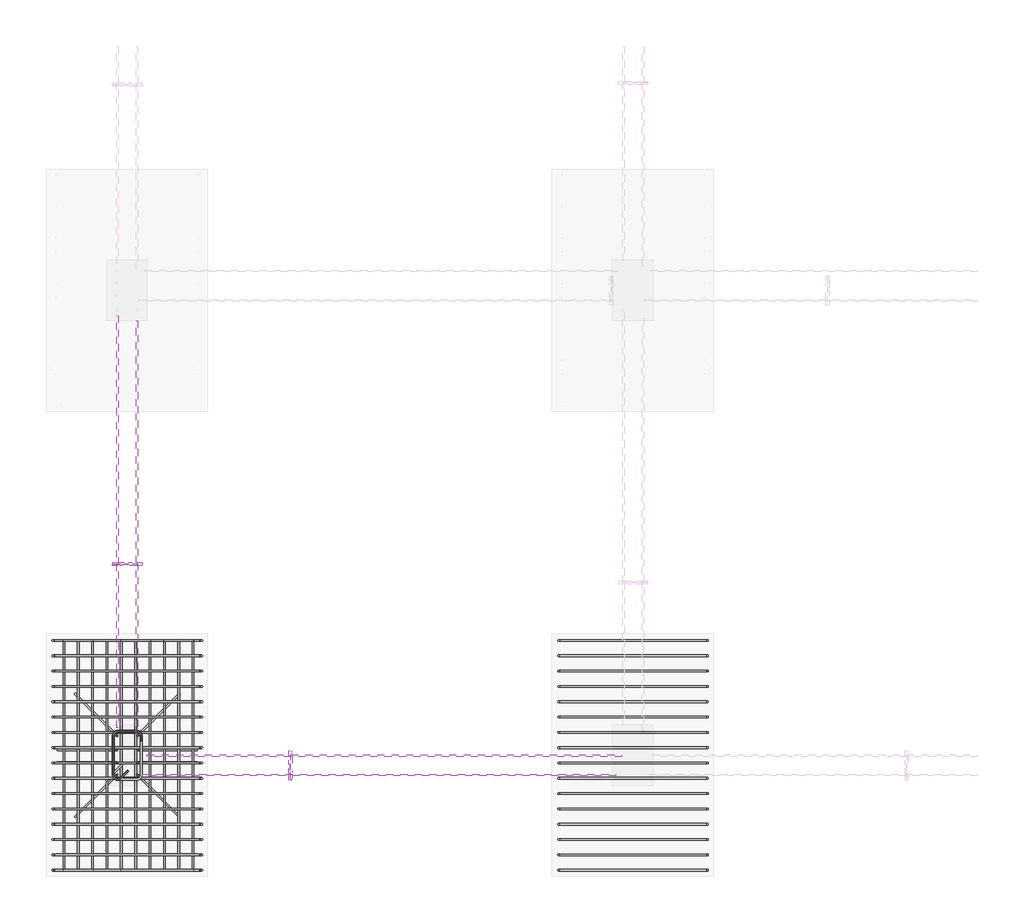
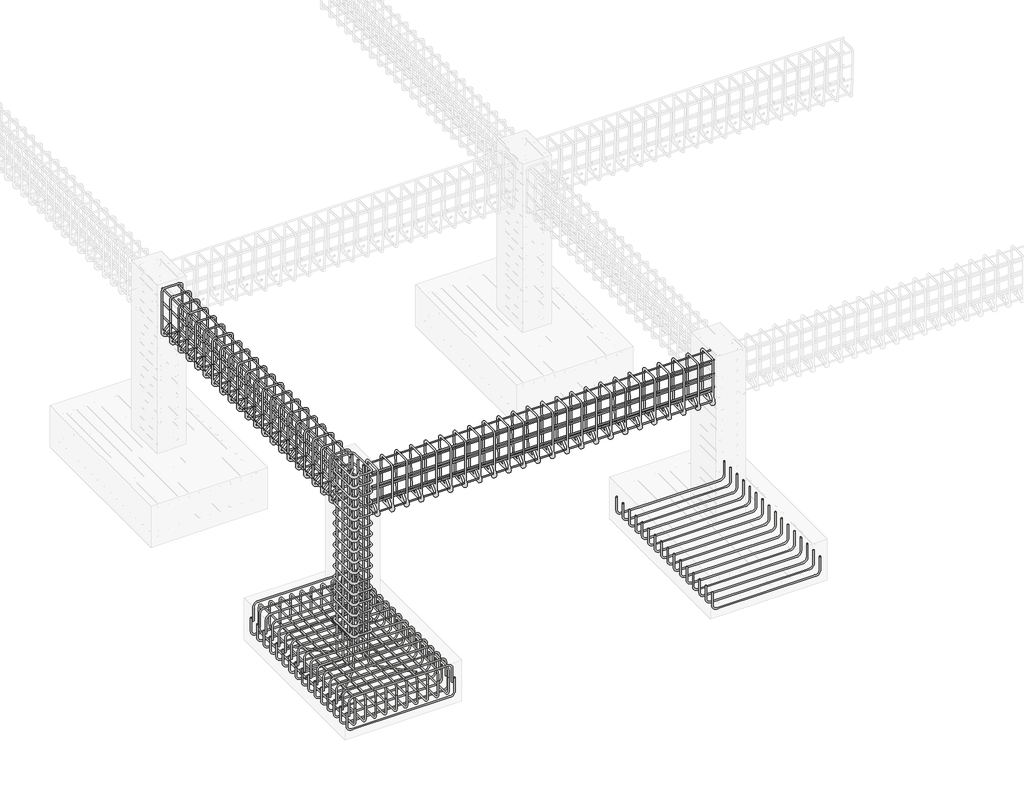
# One storey, part 2 of 20: 18 reinforcing bars.
"""IFC4 building model written with IfcOpenShell, lengths in millimetres."""

from ifc_helpers import new_model, si_unit, point, frame, origin, place, context, project, spatial, polyline, circle_curve, trimmed, segment, composite_curve, source, transform, mapped, element, save
from ifc_brep_helpers import swept_disk

model = new_model("IFC4")

# Units and contexts
model_context = context("Model", 3, world=origin())
ifc_project = project(units=[si_unit("LENGTHUNIT", "METRE", prefix="MILLI")], contexts=[model_context])

# Site, building, storey
site = spatial("IfcSite", under=ifc_project)
building = spatial("IfcBuilding", under=site)
storey = spatial("IfcBuildingStorey", under=building, Elevation=-1828.8)

# Reinforcing bars
placement = place(None, origin())
reinforcing_bar_shape = source(origin(), model_context, "Body", "SolidModel", [
    swept_disk(composite_curve([segment(polyline([(-6417.5912236, -7032.7168637, -2028.4704493), (-6417.5912236, -7032.7168637, -2175.7704493)]), True, "CONTINUOUS"), segment(trimmed(circle_curve(frame((-6371.2412236, -7032.7168637, -2175.7704493), z_axis=(0.0, -1.0, 0.0), x_axis=(-46.350000000000364, 0.0, 0.0)), 46.35), [point((-6417.5912236, -7032.7168637, -2175.7704493))], [point((-6371.2412236, -7032.7168637, -2222.1204493))], True, "CARTESIAN"), True, "CONTINUOUS"), segment(polyline([(-6371.2412236, -7032.7168637, -2222.1204493), (-5356.6412236, -7032.7168637, -2222.1204493)]), True, "CONTINUOUS"), segment(trimmed(circle_curve(frame((-5356.6412236, -7032.7168637, -2175.7704493), z_axis=(0.0, -1.0, 0.0), x_axis=(0.0, 0.0, -46.34999999999991)), 46.35), [point((-5356.6412236, -7032.7168637, -2222.1204493))], [point((-5310.2912236, -7032.7168637, -2175.7704493))], True, "CARTESIAN"), True, "CONTINUOUS"), segment(polyline([(-5310.2912236, -7032.7168637, -2175.7704493), (-5310.2912236, -7032.7168637, -2028.4704493)]), True, "CONTINUOUS")], self_intersect=False), 6.35),
])
element("IfcReinforcingBar", 1, at=placement, inside=storey, context=model_context, shape_type="MappedRepresentation", body=[
    mapped(reinforcing_bar_shape, transform((0.0, 0.0, 0.0), x_axis=(1.0, 0.0, 0.0), y_axis=(0.0, 1.0, 0.0), z_axis=(0.0, 0.0, 1.0))),
    mapped(reinforcing_bar_shape, transform((0.0, 113.82, 0.0), x_axis=(1.0, 0.0, 0.0), y_axis=(0.0, 1.0, 0.0), z_axis=(0.0, 0.0, 1.0))),
    mapped(reinforcing_bar_shape, transform((0.0, 227.64, 0.0), x_axis=(1.0, 0.0, 0.0), y_axis=(0.0, 1.0, 0.0), z_axis=(0.0, 0.0, 1.0))),
    mapped(reinforcing_bar_shape, transform((0.0, 341.46, 0.0), x_axis=(1.0, 0.0, 0.0), y_axis=(0.0, 1.0, 0.0), z_axis=(0.0, 0.0, 1.0))),
    mapped(reinforcing_bar_shape, transform((0.0, 455.28, 0.0), x_axis=(1.0, 0.0, 0.0), y_axis=(0.0, 1.0, 0.0), z_axis=(0.0, 0.0, 1.0))),
    mapped(reinforcing_bar_shape, transform((0.0, 569.1, 0.0), x_axis=(1.0, 0.0, 0.0), y_axis=(0.0, 1.0, 0.0), z_axis=(0.0, 0.0, 1.0))),
    mapped(reinforcing_bar_shape, transform((0.0, 682.92, 0.0), x_axis=(1.0, 0.0, 0.0), y_axis=(0.0, 1.0, 0.0), z_axis=(0.0, 0.0, 1.0))),
    mapped(reinforcing_bar_shape, transform((0.0, 796.74, 0.0), x_axis=(1.0, 0.0, 0.0), y_axis=(0.0, 1.0, 0.0), z_axis=(0.0, 0.0, 1.0))),
    mapped(reinforcing_bar_shape, transform((0.0, 910.56, 0.0), x_axis=(1.0, 0.0, 0.0), y_axis=(0.0, 1.0, 0.0), z_axis=(0.0, 0.0, 1.0))),
    mapped(reinforcing_bar_shape, transform((0.0, 1024.38, 0.0), x_axis=(1.0, 0.0, 0.0), y_axis=(0.0, 1.0, 0.0), z_axis=(0.0, 0.0, 1.0))),
    mapped(reinforcing_bar_shape, transform((0.0, 1138.2, 0.0), x_axis=(1.0, 0.0, 0.0), y_axis=(0.0, 1.0, 0.0), z_axis=(0.0, 0.0, 1.0))),
    mapped(reinforcing_bar_shape, transform((0.0, 1252.02, 0.0), x_axis=(1.0, 0.0, 0.0), y_axis=(0.0, 1.0, 0.0), z_axis=(0.0, 0.0, 1.0))),
    mapped(reinforcing_bar_shape, transform((0.0, 1365.84, 0.0), x_axis=(1.0, 0.0, 0.0), y_axis=(0.0, 1.0, 0.0), z_axis=(0.0, 0.0, 1.0))),
    mapped(reinforcing_bar_shape, transform((0.0, 1479.66, 0.0), x_axis=(1.0, 0.0, 0.0), y_axis=(0.0, 1.0, 0.0), z_axis=(0.0, 0.0, 1.0))),
    mapped(reinforcing_bar_shape, transform((0.0, 1593.48, 0.0), x_axis=(1.0, 0.0, 0.0), y_axis=(0.0, 1.0, 0.0), z_axis=(0.0, 0.0, 1.0))),
    mapped(reinforcing_bar_shape, transform((0.0, 1707.3, 0.0), x_axis=(1.0, 0.0, 0.0), y_axis=(0.0, 1.0, 0.0), z_axis=(0.0, 0.0, 1.0))),
])
reinforcing_bar_2_shape = source(origin(), model_context, "Body", "SolidModel", [
    swept_disk(composite_curve([segment(polyline([(-5334.4655685, -7032.7168637, -2068.8), (-5334.4655685, -7032.7168637, -1921.5)]), True, "CONTINUOUS"), segment(trimmed(circle_curve(frame((-5380.8155685, -7032.7168637, -1921.5), z_axis=(0.0, -1.0, 0.0), x_axis=(46.350000000000364, 0.0, 0.0)), 46.35), [point((-5334.4655685, -7032.7168637, -1921.5))], [point((-5380.8155685, -7032.7168637, -1875.15))], True, "CARTESIAN"), True, "CONTINUOUS"), segment(polyline([(-5380.8155685, -7032.7168637, -1875.15), (-6348.5369603, -7032.7168637, -1875.15)]), True, "CONTINUOUS"), segment(trimmed(circle_curve(frame((-6348.5369603, -7032.7168637, -1921.5), z_axis=(0.0, -1.0, 0.0), x_axis=(0.0, 0.0, 46.34999999999991)), 46.35), [point((-6348.5369603, -7032.7168637, -1875.15))], [point((-6394.8869603, -7032.7168637, -1921.5))], True, "CARTESIAN"), True, "CONTINUOUS"), segment(polyline([(-6394.8869603, -7032.7168637, -1921.5), (-6394.8869603, -7032.7168637, -2068.8)]), True, "CONTINUOUS")], self_intersect=False), 6.35),
])
element("IfcReinforcingBar", 2, at=placement, inside=storey, context=model_context, shape_type="MappedRepresentation", body=[
    mapped(reinforcing_bar_2_shape, transform((0.0, 0.0, 0.0), x_axis=(1.0, 0.0, 0.0), y_axis=(0.0, 1.0, 0.0), z_axis=(0.0, 0.0, 1.0))),
    mapped(reinforcing_bar_2_shape, transform((0.0, 113.82, 0.0), x_axis=(1.0, 0.0, 0.0), y_axis=(0.0, 1.0, 0.0), z_axis=(0.0, 0.0, 1.0))),
    mapped(reinforcing_bar_2_shape, transform((0.0, 227.64, 0.0), x_axis=(1.0, 0.0, 0.0), y_axis=(0.0, 1.0, 0.0), z_axis=(0.0, 0.0, 1.0))),
    mapped(reinforcing_bar_2_shape, transform((0.0, 341.46, 0.0), x_axis=(1.0, 0.0, 0.0), y_axis=(0.0, 1.0, 0.0), z_axis=(0.0, 0.0, 1.0))),
    mapped(reinforcing_bar_2_shape, transform((0.0, 455.28, 0.0), x_axis=(1.0, 0.0, 0.0), y_axis=(0.0, 1.0, 0.0), z_axis=(0.0, 0.0, 1.0))),
    mapped(reinforcing_bar_2_shape, transform((0.0, 569.1, 0.0), x_axis=(1.0, 0.0, 0.0), y_axis=(0.0, 1.0, 0.0), z_axis=(0.0, 0.0, 1.0))),
    mapped(reinforcing_bar_2_shape, transform((0.0, 682.92, 0.0), x_axis=(1.0, 0.0, 0.0), y_axis=(0.0, 1.0, 0.0), z_axis=(0.0, 0.0, 1.0))),
    mapped(reinforcing_bar_2_shape, transform((0.0, 796.74, 0.0), x_axis=(1.0, 0.0, 0.0), y_axis=(0.0, 1.0, 0.0), z_axis=(0.0, 0.0, 1.0))),
    mapped(reinforcing_bar_2_shape, transform((0.0, 910.56, 0.0), x_axis=(1.0, 0.0, 0.0), y_axis=(0.0, 1.0, 0.0), z_axis=(0.0, 0.0, 1.0))),
    mapped(reinforcing_bar_2_shape, transform((0.0, 1024.38, 0.0), x_axis=(1.0, 0.0, 0.0), y_axis=(0.0, 1.0, 0.0), z_axis=(0.0, 0.0, 1.0))),
    mapped(reinforcing_bar_2_shape, transform((0.0, 1138.2, 0.0), x_axis=(1.0, 0.0, 0.0), y_axis=(0.0, 1.0, 0.0), z_axis=(0.0, 0.0, 1.0))),
    mapped(reinforcing_bar_2_shape, transform((0.0, 1252.02, 0.0), x_axis=(1.0, 0.0, 0.0), y_axis=(0.0, 1.0, 0.0), z_axis=(0.0, 0.0, 1.0))),
    mapped(reinforcing_bar_2_shape, transform((0.0, 1365.84, 0.0), x_axis=(1.0, 0.0, 0.0), y_axis=(0.0, 1.0, 0.0), z_axis=(0.0, 0.0, 1.0))),
    mapped(reinforcing_bar_2_shape, transform((0.0, 1479.66, 0.0), x_axis=(1.0, 0.0, 0.0), y_axis=(0.0, 1.0, 0.0), z_axis=(0.0, 0.0, 1.0))),
    mapped(reinforcing_bar_2_shape, transform((0.0, 1593.48, 0.0), x_axis=(1.0, 0.0, 0.0), y_axis=(0.0, 1.0, 0.0), z_axis=(0.0, 0.0, 1.0))),
    mapped(reinforcing_bar_2_shape, transform((0.0, 1707.3, 0.0), x_axis=(1.0, 0.0, 0.0), y_axis=(0.0, 1.0, 0.0), z_axis=(0.0, 0.0, 1.0))),
])
reinforcing_bar_3_shape = source(origin(), model_context, "Body", "SolidModel", [
    swept_disk(composite_curve([segment(polyline([(-5374.0329187, -7032.7168637, -2008.6504502), (-5374.0329187, -7032.7168637, -2155.9504502)]), True, "CONTINUOUS"), segment(trimmed(circle_curve(frame((-5374.0329187, -6986.3668637, -2155.9504502), z_axis=(1.0, 0.0, 0.0), x_axis=(0.0, -46.350000000000364, 0.0)), 46.35), [point((-5374.0329187, -7032.7168637, -2155.9504502))], [point((-5374.0329187, -6986.3668637, -2202.3004502))], True, "CARTESIAN"), True, "CONTINUOUS"), segment(polyline([(-5374.0329187, -6986.3668637, -2202.3004502), (-5374.0329187, -5371.7668637, -2202.3004502)]), True, "CONTINUOUS"), segment(trimmed(circle_curve(frame((-5374.0329187, -5371.7668637, -2155.9504502), z_axis=(1.0, 0.0, 0.0), x_axis=(0.0, 0.0, -46.34999999999991)), 46.35), [point((-5374.0329187, -5371.7668637, -2202.3004502))], [point((-5374.0329187, -5325.4168637, -2155.9504502))], True, "CARTESIAN"), True, "CONTINUOUS"), segment(polyline([(-5374.0329187, -5325.4168637, -2155.9504502), (-5374.0329187, -5325.4168637, -2008.6504502)]), True, "CONTINUOUS")], self_intersect=False), 6.35),
])
element("IfcReinforcingBar", 3, at=placement, inside=storey, context=model_context, shape_type="MappedRepresentation", body=[
    mapped(reinforcing_bar_3_shape, transform((0.0, 0.0, 0.0), x_axis=(1.0, 0.0, 0.0), y_axis=(0.0, 1.0, 0.0), z_axis=(0.0, 0.0, 1.0))),
    mapped(reinforcing_bar_3_shape, transform((-106.7711398, 0.0, 0.0), x_axis=(1.0, 0.0, 0.0), y_axis=(0.0, 1.0, 0.0), z_axis=(0.0, 0.0, 1.0))),
    mapped(reinforcing_bar_3_shape, transform((-213.5422797, 0.0, 0.0), x_axis=(1.0, 0.0, 0.0), y_axis=(0.0, 1.0, 0.0), z_axis=(0.0, 0.0, 1.0))),
    mapped(reinforcing_bar_3_shape, transform((-320.3134195, 0.0, 0.0), x_axis=(1.0, 0.0, 0.0), y_axis=(0.0, 1.0, 0.0), z_axis=(0.0, 0.0, 1.0))),
    mapped(reinforcing_bar_3_shape, transform((-427.0845593, 0.0, 0.0), x_axis=(1.0, 0.0, 0.0), y_axis=(0.0, 1.0, 0.0), z_axis=(0.0, 0.0, 1.0))),
    mapped(reinforcing_bar_3_shape, transform((-533.8556992, 0.0, 0.0), x_axis=(1.0, 0.0, 0.0), y_axis=(0.0, 1.0, 0.0), z_axis=(0.0, 0.0, 1.0))),
    mapped(reinforcing_bar_3_shape, transform((-640.626839, 0.0, 0.0), x_axis=(1.0, 0.0, 0.0), y_axis=(0.0, 1.0, 0.0), z_axis=(0.0, 0.0, 1.0))),
    mapped(reinforcing_bar_3_shape, transform((-747.3979788, 0.0, 0.0), x_axis=(1.0, 0.0, 0.0), y_axis=(0.0, 1.0, 0.0), z_axis=(0.0, 0.0, 1.0))),
    mapped(reinforcing_bar_3_shape, transform((-854.1691187, 0.0, 0.0), x_axis=(1.0, 0.0, 0.0), y_axis=(0.0, 1.0, 0.0), z_axis=(0.0, 0.0, 1.0))),
    mapped(reinforcing_bar_3_shape, transform((-960.9402585, 0.0, 0.0), x_axis=(1.0, 0.0, 0.0), y_axis=(0.0, 1.0, 0.0), z_axis=(0.0, 0.0, 1.0))),
])
reinforcing_bar_4_shape = source(origin(), model_context, "Body", "SolidModel", [
    swept_disk(composite_curve([segment(polyline([(-6334.9731772, -7032.7168637, -2088.5147466), (-6334.9731772, -7032.7168637, -1941.2147466)]), True, "CONTINUOUS"), segment(trimmed(circle_curve(frame((-6334.9731772, -6986.3668637, -1941.2147466), z_axis=(-1.0, 0.0, 0.0), x_axis=(0.0, -46.350000000000364, 0.0)), 46.35), [point((-6334.9731772, -7032.7168637, -1941.2147466))], [point((-6334.9731772, -6986.3668637, -1894.8647466))], True, "CARTESIAN"), True, "CONTINUOUS"), segment(polyline([(-6334.9731772, -6986.3668637, -1894.8647466), (-6334.9731772, -5371.7668637, -1894.8647466)]), True, "CONTINUOUS"), segment(trimmed(circle_curve(frame((-6334.9731772, -5371.7668637, -1941.2147466), z_axis=(-1.0, 0.0, 0.0), x_axis=(0.0, 0.0, 46.34999999999991)), 46.35), [point((-6334.9731772, -5371.7668637, -1894.8647466))], [point((-6334.9731772, -5325.4168637, -1941.2147466))], True, "CARTESIAN"), True, "CONTINUOUS"), segment(polyline([(-6334.9731772, -5325.4168637, -1941.2147466), (-6334.9731772, -5325.4168637, -2088.5147466)]), True, "CONTINUOUS")], self_intersect=False), 6.35),
])
element("IfcReinforcingBar", 4, at=placement, inside=storey, context=model_context, shape_type="MappedRepresentation", body=[
    mapped(reinforcing_bar_4_shape, transform((0.0, 0.0, 0.0), x_axis=(1.0, 0.0, 0.0), y_axis=(0.0, 1.0, 0.0), z_axis=(0.0, 0.0, 1.0))),
    mapped(reinforcing_bar_4_shape, transform((106.7711398, 0.0, 0.0), x_axis=(1.0, 0.0, 0.0), y_axis=(0.0, 1.0, 0.0), z_axis=(0.0, 0.0, 1.0))),
    mapped(reinforcing_bar_4_shape, transform((213.5422797, 0.0, 0.0), x_axis=(1.0, 0.0, 0.0), y_axis=(0.0, 1.0, 0.0), z_axis=(0.0, 0.0, 1.0))),
    mapped(reinforcing_bar_4_shape, transform((320.3134195, 0.0, 0.0), x_axis=(1.0, 0.0, 0.0), y_axis=(0.0, 1.0, 0.0), z_axis=(0.0, 0.0, 1.0))),
    mapped(reinforcing_bar_4_shape, transform((427.0845593, 0.0, 0.0), x_axis=(1.0, 0.0, 0.0), y_axis=(0.0, 1.0, 0.0), z_axis=(0.0, 0.0, 1.0))),
    mapped(reinforcing_bar_4_shape, transform((533.8556992, 0.0, 0.0), x_axis=(1.0, 0.0, 0.0), y_axis=(0.0, 1.0, 0.0), z_axis=(0.0, 0.0, 1.0))),
    mapped(reinforcing_bar_4_shape, transform((640.626839, 0.0, 0.0), x_axis=(1.0, 0.0, 0.0), y_axis=(0.0, 1.0, 0.0), z_axis=(0.0, 0.0, 1.0))),
    mapped(reinforcing_bar_4_shape, transform((747.3979788, 0.0, 0.0), x_axis=(1.0, 0.0, 0.0), y_axis=(0.0, 1.0, 0.0), z_axis=(0.0, 0.0, 1.0))),
    mapped(reinforcing_bar_4_shape, transform((854.1691187, 0.0, 0.0), x_axis=(1.0, 0.0, 0.0), y_axis=(0.0, 1.0, 0.0), z_axis=(0.0, 0.0, 1.0))),
    mapped(reinforcing_bar_4_shape, transform((960.9402585, 0.0, 0.0), x_axis=(1.0, 0.0, 0.0), y_axis=(0.0, 1.0, 0.0), z_axis=(0.0, 0.0, 1.0))),
])
reinforcing_bar_5_shape = source(origin(), model_context, "Body", "SolidModel", [
    swept_disk(composite_curve([segment(polyline([(-2656.4360107, -7032.7168637, -2028.4704493), (-2656.4360107, -7032.7168637, -2175.7704493)]), True, "CONTINUOUS"), segment(trimmed(circle_curve(frame((-2610.0860107, -7032.7168637, -2175.7704493), z_axis=(0.0, -1.0, 0.0), x_axis=(-46.350000000000364, 0.0, 0.0)), 46.35), [point((-2656.4360107, -7032.7168637, -2175.7704493))], [point((-2610.0860107, -7032.7168637, -2222.1204493))], True, "CARTESIAN"), True, "CONTINUOUS"), segment(polyline([(-2610.0860107, -7032.7168637, -2222.1204493), (-1595.4860107, -7032.7168637, -2222.1204493)]), True, "CONTINUOUS"), segment(trimmed(circle_curve(frame((-1595.4860107, -7032.7168637, -2175.7704493), z_axis=(0.0, -1.0, 0.0), x_axis=(0.0, 0.0, -46.34999999999991)), 46.35), [point((-1595.4860107, -7032.7168637, -2222.1204493))], [point((-1549.1360107, -7032.7168637, -2175.7704493))], True, "CARTESIAN"), True, "CONTINUOUS"), segment(polyline([(-1549.1360107, -7032.7168637, -2175.7704493), (-1549.1360107, -7032.7168637, -2028.4704493)]), True, "CONTINUOUS")], self_intersect=False), 6.35),
])
element("IfcReinforcingBar", 5, at=placement, inside=storey, context=model_context, shape_type="MappedRepresentation", body=[
    mapped(reinforcing_bar_5_shape, transform((0.0, 0.0, 0.0), x_axis=(1.0, 0.0, 0.0), y_axis=(0.0, 1.0, 0.0), z_axis=(0.0, 0.0, 1.0))),
    mapped(reinforcing_bar_5_shape, transform((0.0, 113.82, 0.0), x_axis=(1.0, 0.0, 0.0), y_axis=(0.0, 1.0, 0.0), z_axis=(0.0, 0.0, 1.0))),
    mapped(reinforcing_bar_5_shape, transform((0.0, 227.64, 0.0), x_axis=(1.0, 0.0, 0.0), y_axis=(0.0, 1.0, 0.0), z_axis=(0.0, 0.0, 1.0))),
    mapped(reinforcing_bar_5_shape, transform((0.0, 341.46, 0.0), x_axis=(1.0, 0.0, 0.0), y_axis=(0.0, 1.0, 0.0), z_axis=(0.0, 0.0, 1.0))),
    mapped(reinforcing_bar_5_shape, transform((0.0, 455.28, 0.0), x_axis=(1.0, 0.0, 0.0), y_axis=(0.0, 1.0, 0.0), z_axis=(0.0, 0.0, 1.0))),
    mapped(reinforcing_bar_5_shape, transform((0.0, 569.1, 0.0), x_axis=(1.0, 0.0, 0.0), y_axis=(0.0, 1.0, 0.0), z_axis=(0.0, 0.0, 1.0))),
    mapped(reinforcing_bar_5_shape, transform((0.0, 682.92, 0.0), x_axis=(1.0, 0.0, 0.0), y_axis=(0.0, 1.0, 0.0), z_axis=(0.0, 0.0, 1.0))),
    mapped(reinforcing_bar_5_shape, transform((0.0, 796.74, 0.0), x_axis=(1.0, 0.0, 0.0), y_axis=(0.0, 1.0, 0.0), z_axis=(0.0, 0.0, 1.0))),
    mapped(reinforcing_bar_5_shape, transform((0.0, 910.56, 0.0), x_axis=(1.0, 0.0, 0.0), y_axis=(0.0, 1.0, 0.0), z_axis=(0.0, 0.0, 1.0))),
    mapped(reinforcing_bar_5_shape, transform((0.0, 1024.38, 0.0), x_axis=(1.0, 0.0, 0.0), y_axis=(0.0, 1.0, 0.0), z_axis=(0.0, 0.0, 1.0))),
    mapped(reinforcing_bar_5_shape, transform((0.0, 1138.2, 0.0), x_axis=(1.0, 0.0, 0.0), y_axis=(0.0, 1.0, 0.0), z_axis=(0.0, 0.0, 1.0))),
    mapped(reinforcing_bar_5_shape, transform((0.0, 1252.02, 0.0), x_axis=(1.0, 0.0, 0.0), y_axis=(0.0, 1.0, 0.0), z_axis=(0.0, 0.0, 1.0))),
    mapped(reinforcing_bar_5_shape, transform((0.0, 1365.84, 0.0), x_axis=(1.0, 0.0, 0.0), y_axis=(0.0, 1.0, 0.0), z_axis=(0.0, 0.0, 1.0))),
    mapped(reinforcing_bar_5_shape, transform((0.0, 1479.66, 0.0), x_axis=(1.0, 0.0, 0.0), y_axis=(0.0, 1.0, 0.0), z_axis=(0.0, 0.0, 1.0))),
    mapped(reinforcing_bar_5_shape, transform((0.0, 1593.48, 0.0), x_axis=(1.0, 0.0, 0.0), y_axis=(0.0, 1.0, 0.0), z_axis=(0.0, 0.0, 1.0))),
    mapped(reinforcing_bar_5_shape, transform((0.0, 1707.3, 0.0), x_axis=(1.0, 0.0, 0.0), y_axis=(0.0, 1.0, 0.0), z_axis=(0.0, 0.0, 1.0))),
])
reinforcing_bar_6_shape = source(origin(), model_context, "Body", "SolidModel", [
    swept_disk(composite_curve([segment(polyline([(-5858.3298631, -6292.7910983, -46.35), (-5914.073426, -6348.5346613, -46.35)]), True, "CONTINUOUS"), segment(trimmed(circle_curve(frame((-5936.2412236, -6326.3668637, -46.35), z_axis=(0.0, 0.0, -1.0), x_axis=(22.167797600000085, -22.167797600000085, 0.0)), 31.35), [point((-5914.073426, -6348.5346613, -46.35))], [point((-5967.5912236, -6326.3668637, -46.35))], True, "CARTESIAN"), True, "CONTINUOUS"), segment(polyline([(-5967.5912236, -6326.3668637, -46.35), (-5967.5912236, -6031.7668637, -46.35)]), True, "CONTINUOUS"), segment(trimmed(circle_curve(frame((-5936.2412236, -6031.7668637, -46.35), z_axis=(0.0, 0.0, -1.0), x_axis=(-31.350000000000364, 0.0, 0.0)), 31.35), [point((-5967.5912236, -6031.7668637, -46.35))], [point((-5936.2412236, -6000.4168637, -46.35))], True, "CARTESIAN"), True, "CONTINUOUS"), segment(polyline([(-5936.2412236, -6000.4168637, -46.35), (-5791.6412236, -6000.4168637, -46.35)]), True, "CONTINUOUS"), segment(trimmed(circle_curve(frame((-5791.6412236, -6031.7470786, -45.2363875), z_axis=(0.0, -0.035521928334481916, -0.9993688971583016), x_axis=(0.0, 31.3302149000001, -1.1136125000000021)), 31.35), [point((-5791.6412236, -6000.4168637, -46.35))], [point((-5760.2912236, -6031.7470786, -45.2363875))], True, "CARTESIAN"), True, "CONTINUOUS"), segment(polyline([(-5760.2912236, -6031.7470786, -45.2363875), (-5760.2912236, -6326.3866488, -34.7636125)]), True, "CONTINUOUS"), segment(trimmed(circle_curve(frame((-5791.6412236, -6326.3866488, -34.7636125), z_axis=(0.0, -0.035521928334481916, -0.9993688971583016), x_axis=(31.349999999999454, 0.0, 0.0)), 31.35), [point((-5760.2912236, -6326.3866488, -34.7636125))], [point((-5791.6412236, -6357.7168637, -33.65))], True, "CARTESIAN"), True, "CONTINUOUS"), segment(polyline([(-5791.6412236, -6357.7168637, -33.65), (-5936.2412236, -6357.7168637, -33.65)]), True, "CONTINUOUS"), segment(trimmed(circle_curve(frame((-5936.2412236, -6326.3668637, -33.65), z_axis=(0.0, 0.0, -1.0), x_axis=(0.0, -31.350000000000364, 0.0)), 31.35), [point((-5936.2412236, -6357.7168637, -33.65))], [point((-5958.4090212, -6304.1990661, -33.65))], True, "CARTESIAN"), True, "CONTINUOUS"), segment(polyline([(-5958.4090212, -6304.1990661, -33.65), (-5902.6654583, -6248.4555031, -33.65)]), True, "CONTINUOUS")], self_intersect=False), 6.35),
])
element("IfcReinforcingBar", 6, at=placement, inside=storey, context=model_context, shape_type="MappedRepresentation", body=[
    mapped(reinforcing_bar_6_shape, transform((0.0, 0.0, 0.0), x_axis=(1.0, 0.0, 0.0), y_axis=(0.0, 1.0, 0.0), z_axis=(0.0, 0.0, 1.0))),
    mapped(reinforcing_bar_6_shape, transform((0.0, 0.0, -115.74), x_axis=(1.0, 0.0, 0.0), y_axis=(0.0, 1.0, 0.0), z_axis=(0.0, 0.0, 1.0))),
    mapped(reinforcing_bar_6_shape, transform((0.0, 0.0, -231.48), x_axis=(1.0, 0.0, 0.0), y_axis=(0.0, 1.0, 0.0), z_axis=(0.0, 0.0, 1.0))),
    mapped(reinforcing_bar_6_shape, transform((0.0, 0.0, -347.22), x_axis=(1.0, 0.0, 0.0), y_axis=(0.0, 1.0, 0.0), z_axis=(0.0, 0.0, 1.0))),
    mapped(reinforcing_bar_6_shape, transform((0.0, 0.0, -462.96), x_axis=(1.0, 0.0, 0.0), y_axis=(0.0, 1.0, 0.0), z_axis=(0.0, 0.0, 1.0))),
    mapped(reinforcing_bar_6_shape, transform((0.0, 0.0, -578.7), x_axis=(1.0, 0.0, 0.0), y_axis=(0.0, 1.0, 0.0), z_axis=(0.0, 0.0, 1.0))),
    mapped(reinforcing_bar_6_shape, transform((0.0, 0.0, -694.44), x_axis=(1.0, 0.0, 0.0), y_axis=(0.0, 1.0, 0.0), z_axis=(0.0, 0.0, 1.0))),
    mapped(reinforcing_bar_6_shape, transform((0.0, 0.0, -810.18), x_axis=(1.0, 0.0, 0.0), y_axis=(0.0, 1.0, 0.0), z_axis=(0.0, 0.0, 1.0))),
    mapped(reinforcing_bar_6_shape, transform((0.0, 0.0, -925.92), x_axis=(1.0, 0.0, 0.0), y_axis=(0.0, 1.0, 0.0), z_axis=(0.0, 0.0, 1.0))),
    mapped(reinforcing_bar_6_shape, transform((0.0, 0.0, -1041.66), x_axis=(1.0, 0.0, 0.0), y_axis=(0.0, 1.0, 0.0), z_axis=(0.0, 0.0, 1.0))),
    mapped(reinforcing_bar_6_shape, transform((0.0, 0.0, -1157.4), x_axis=(1.0, 0.0, 0.0), y_axis=(0.0, 1.0, 0.0), z_axis=(0.0, 0.0, 1.0))),
    mapped(reinforcing_bar_6_shape, transform((0.0, 0.0, -1273.14), x_axis=(1.0, 0.0, 0.0), y_axis=(0.0, 1.0, 0.0), z_axis=(0.0, 0.0, 1.0))),
    mapped(reinforcing_bar_6_shape, transform((0.0, 0.0, -1388.88), x_axis=(1.0, 0.0, 0.0), y_axis=(0.0, 1.0, 0.0), z_axis=(0.0, 0.0, 1.0))),
    mapped(reinforcing_bar_6_shape, transform((0.0, 0.0, -1504.62), x_axis=(1.0, 0.0, 0.0), y_axis=(0.0, 1.0, 0.0), z_axis=(0.0, 0.0, 1.0))),
    mapped(reinforcing_bar_6_shape, transform((0.0, 0.0, -1620.36), x_axis=(1.0, 0.0, 0.0), y_axis=(0.0, 1.0, 0.0), z_axis=(0.0, 0.0, 1.0))),
    mapped(reinforcing_bar_6_shape, transform((0.0, 0.0, -1736.1), x_axis=(1.0, 0.0, 0.0), y_axis=(0.0, 1.0, 0.0), z_axis=(0.0, 0.0, 1.0))),
])
reinforcing_bar_7_shape = source(origin(), model_context, "Body", "SolidModel", [
    swept_disk(composite_curve([segment(polyline([(-5343.4123372, -6232.7428863, -2151.8747939), (-5740.4296686, -6232.7428863, -2151.8747939)]), True, "CONTINUOUS"), segment(trimmed(circle_curve(frame((-5740.4296686, -6232.7428863, -2105.5247939), z_axis=(0.0, 1.0, 0.0), x_axis=(0.0, 0.0, -46.34999999999991)), 46.35), [point((-5740.4296686, -6232.7428863, -2151.8747939))], [point((-5786.7796686, -6232.7428863, -2105.5247939))], True, "CARTESIAN"), True, "CONTINUOUS"), segment(polyline([(-5786.7796686, -6232.7428863, -2105.5247939), (-5786.7796686, -6232.7428863, -40.0)]), True, "CONTINUOUS")], self_intersect=False), 6.35),
])
element("IfcReinforcingBar", 7, at=placement, inside=storey, context=model_context, shape_type="MappedRepresentation", body=[
    mapped(reinforcing_bar_7_shape, transform((0.0, 0.0, 0.0), x_axis=(1.0, 0.0, 0.0), y_axis=(0.0, 1.0, 0.0), z_axis=(0.0, 0.0, 1.0))),
    mapped(reinforcing_bar_7_shape, transform((0.0, 93.9182821, 0.0), x_axis=(1.0, 0.0, 0.0), y_axis=(0.0, 1.0, 0.0), z_axis=(0.0, 0.0, 1.0))),
])
element("IfcReinforcingBar", 8, at=placement, inside=storey, context=model_context, shape_type="SolidModel", body=[
    swept_disk(composite_curve([segment(polyline([(-5473.271622, -5719.5629186, -2151.8747939), (-5754.0052693, -6000.2965659, -2151.8747939)]), True, "CONTINUOUS"), segment(trimmed(circle_curve(frame((-5754.0052693, -6000.2965659, -2105.5247939), z_axis=(-0.7071067811865442, 0.7071067811865509, 0.0), x_axis=(0.0, 0.0, -46.34999999999991)), 46.35), [point((-5754.0052693, -6000.2965659, -2151.8747939))], [point((-5786.7796686, -6033.0709652, -2105.5247939))], True, "CARTESIAN"), True, "CONTINUOUS"), segment(polyline([(-5786.7796686, -6033.0709652, -2105.5247939), (-5786.7796686, -6033.0709652, -40.0)]), True, "CONTINUOUS")], self_intersect=False), 6.35),
])
element("IfcReinforcingBar", 9, at=placement, inside=storey, context=model_context, shape_type="SolidModel", body=[
    swept_disk(composite_curve([segment(polyline([(-6254.6108252, -5719.5629186, -2151.8747939), (-5973.877178, -6000.2965659, -2151.8747939)]), True, "CONTINUOUS"), segment(trimmed(circle_curve(frame((-5973.877178, -6000.2965659, -2105.5247939), z_axis=(-0.7071067811865442, -0.7071067811865509, 0.0), x_axis=(0.0, 0.0, -46.34999999999991)), 46.35), [point((-5973.877178, -6000.2965659, -2151.8747939))], [point((-5941.1027787, -6033.0709652, -2105.5247939))], True, "CARTESIAN"), True, "CONTINUOUS"), segment(polyline([(-5941.1027787, -6033.0709652, -2105.5247939), (-5941.1027787, -6033.0709652, -40.0)]), True, "CONTINUOUS")], self_intersect=False), 6.35),
])
element("IfcReinforcingBar", 10, at=placement, inside=storey, context=model_context, shape_type="SolidModel", body=[
    swept_disk(composite_curve([segment(polyline([(-5473.271622, -6638.5708088, -2151.8747939), (-5754.0052693, -6357.8371615, -2151.8747939)]), True, "CONTINUOUS"), segment(trimmed(circle_curve(frame((-5754.0052693, -6357.8371615, -2105.5247939), z_axis=(0.7071067811865442, 0.7071067811865509, 0.0), x_axis=(0.0, 0.0, -46.34999999999991)), 46.35), [point((-5754.0052693, -6357.8371615, -2151.8747939))], [point((-5786.7796686, -6325.0627622, -2105.5247939))], True, "CARTESIAN"), True, "CONTINUOUS"), segment(polyline([(-5786.7796686, -6325.0627622, -2105.5247939), (-5786.7796686, -6325.0627622, -40.0)]), True, "CONTINUOUS")], self_intersect=False), 6.35),
])
element("IfcReinforcingBar", 11, at=placement, inside=storey, context=model_context, shape_type="SolidModel", body=[
    swept_disk(composite_curve([segment(polyline([(-6254.6108252, -6638.5708088, -2151.8747939), (-5973.877178, -6357.8371615, -2151.8747939)]), True, "CONTINUOUS"), segment(trimmed(circle_curve(frame((-5973.877178, -6357.8371615, -2105.5247939), z_axis=(0.7071067811865442, -0.7071067811865509, 0.0), x_axis=(0.0, 0.0, -46.34999999999991)), 46.35), [point((-5973.877178, -6357.8371615, -2151.8747939))], [point((-5941.1027787, -6325.0627622, -2105.5247939))], True, "CARTESIAN"), True, "CONTINUOUS"), segment(polyline([(-5941.1027787, -6325.0627622, -2105.5247939), (-5941.1027787, -6325.0627622, -40.0)]), True, "CONTINUOUS")], self_intersect=False), 6.35),
])
reinforcing_bar_8_shape = source(origin(), model_context, "Body", "SolidModel", [
    swept_disk(composite_curve([segment(polyline([(-6384.4701101, -6232.7428863, -2151.8747939), (-5987.4527787, -6232.7428863, -2151.8747939)]), True, "CONTINUOUS"), segment(trimmed(circle_curve(frame((-5987.4527787, -6232.7428863, -2105.5247939), z_axis=(0.0, -1.0, 0.0), x_axis=(0.0, 0.0, -46.34999999999991)), 46.35), [point((-5987.4527787, -6232.7428863, -2151.8747939))], [point((-5941.1027787, -6232.7428863, -2105.5247939))], True, "CARTESIAN"), True, "CONTINUOUS"), segment(polyline([(-5941.1027787, -6232.7428863, -2105.5247939), (-5941.1027787, -6232.7428863, -40.0)]), True, "CONTINUOUS")], self_intersect=False), 6.35),
])
element("IfcReinforcingBar", 12, at=placement, inside=storey, context=model_context, shape_type="MappedRepresentation", body=[
    mapped(reinforcing_bar_8_shape, transform((0.0, 0.0, 0.0), x_axis=(1.0, 0.0, 0.0), y_axis=(0.0, 1.0, 0.0), z_axis=(0.0, 0.0, 1.0))),
    mapped(reinforcing_bar_8_shape, transform((0.0, 93.9182821, 0.0), x_axis=(1.0, 0.0, 0.0), y_axis=(0.0, 1.0, 0.0), z_axis=(0.0, 0.0, 1.0))),
])
reinforcing_bar_9_shape = source(origin(), model_context, "Body", "SolidModel", [
    swept_disk(composite_curve([segment(polyline([(-5858.3298631, -5947.7168643, -488.7242346), (-5914.073426, -5947.7168643, -544.4677976)]), True, "CONTINUOUS"), segment(trimmed(circle_curve(frame((-5936.2412236, -5947.7168643, -522.3), z_axis=(0.0, 1.0, 0.0), x_axis=(22.167797600000085, 0.0, -22.167797600000085)), 31.35), [point((-5914.073426, -5947.7168643, -544.4677976))], [point((-5967.5912236, -5947.7168643, -522.3))], True, "CARTESIAN"), True, "CONTINUOUS"), segment(polyline([(-5967.5912236, -5947.7168643, -522.3), (-5967.5912236, -5947.7168643, -77.7)]), True, "CONTINUOUS"), segment(trimmed(circle_curve(frame((-5936.2412236, -5947.7168643, -77.7), z_axis=(0.0, 1.0, 0.0), x_axis=(-31.350000000000364, 0.0, 0.0)), 31.35), [point((-5967.5912236, -5947.7168643, -77.7))], [point((-5936.2412236, -5947.7168643, -46.35))], True, "CARTESIAN"), True, "CONTINUOUS"), segment(polyline([(-5936.2412236, -5947.7168643, -46.35), (-5791.6412236, -5947.7168643, -46.35)]), True, "CONTINUOUS"), segment(trimmed(circle_curve(frame((-5791.6412236, -5948.5014499, -77.6901807), z_axis=(0.0, 0.9996867842138424, -0.025026655153786322), x_axis=(0.0, 0.7845855999994455, 31.340180699999998)), 31.35), [point((-5791.6412236, -5947.7168643, -46.35))], [point((-5760.2912236, -5948.5014499, -77.6901807))], True, "CARTESIAN"), True, "CONTINUOUS"), segment(polyline([(-5760.2912236, -5948.5014499, -77.6901807), (-5760.2912236, -5959.6322786, -522.3098193)]), True, "CONTINUOUS"), segment(trimmed(circle_curve(frame((-5791.6412236, -5959.6322786, -522.3098193), z_axis=(0.0, 0.9996867842138424, -0.025026655153786322), x_axis=(31.349999999999454, 0.0, 0.0)), 31.35), [point((-5760.2912236, -5959.6322786, -522.3098193))], [point((-5791.6412236, -5960.4168643, -553.65))], True, "CARTESIAN"), True, "CONTINUOUS"), segment(polyline([(-5791.6412236, -5960.4168643, -553.65), (-5936.2412236, -5960.4168643, -553.65)]), True, "CONTINUOUS"), segment(trimmed(circle_curve(frame((-5936.2412236, -5960.4168643, -522.3), z_axis=(0.0, 1.0, 0.0), x_axis=(0.0, 0.0, -31.350000000000023)), 31.35), [point((-5936.2412236, -5960.4168643, -553.65))], [point((-5958.4090212, -5960.4168643, -500.1322024))], True, "CARTESIAN"), True, "CONTINUOUS"), segment(polyline([(-5958.4090212, -5960.4168643, -500.1322024), (-5902.6654583, -5960.4168643, -444.3886395)]), True, "CONTINUOUS")], self_intersect=False), 6.35),
])
element("IfcReinforcingBar", 13, at=placement, inside=storey, context=model_context, shape_type="MappedRepresentation", body=[
    mapped(reinforcing_bar_9_shape, transform((0.0, 0.0, 0.0), x_axis=(1.0, 0.0, 0.0), y_axis=(0.0, 1.0, 0.0), z_axis=(0.0, 0.0, 1.0))),
    mapped(reinforcing_bar_9_shape, transform((0.0, 149.585, 0.0), x_axis=(1.0, 0.0, 0.0), y_axis=(0.0, 1.0, 0.0), z_axis=(0.0, 0.0, 1.0))),
    mapped(reinforcing_bar_9_shape, transform((0.0, 299.1700001, 0.0), x_axis=(1.0, 0.0, 0.0), y_axis=(0.0, 1.0, 0.0), z_axis=(0.0, 0.0, 1.0))),
    mapped(reinforcing_bar_9_shape, transform((0.0, 448.7550001, 0.0), x_axis=(1.0, 0.0, 0.0), y_axis=(0.0, 1.0, 0.0), z_axis=(0.0, 0.0, 1.0))),
    mapped(reinforcing_bar_9_shape, transform((0.0, 598.3400001, 0.0), x_axis=(1.0, 0.0, 0.0), y_axis=(0.0, 1.0, 0.0), z_axis=(0.0, 0.0, 1.0))),
    mapped(reinforcing_bar_9_shape, transform((0.0, 747.9250002, 0.0), x_axis=(1.0, 0.0, 0.0), y_axis=(0.0, 1.0, 0.0), z_axis=(0.0, 0.0, 1.0))),
    mapped(reinforcing_bar_9_shape, transform((0.0, 897.5100002, 0.0), x_axis=(1.0, 0.0, 0.0), y_axis=(0.0, 1.0, 0.0), z_axis=(0.0, 0.0, 1.0))),
    mapped(reinforcing_bar_9_shape, transform((0.0, 1047.0950002, 0.0), x_axis=(1.0, 0.0, 0.0), y_axis=(0.0, 1.0, 0.0), z_axis=(0.0, 0.0, 1.0))),
    mapped(reinforcing_bar_9_shape, transform((0.0, 1196.6800002, 0.0), x_axis=(1.0, 0.0, 0.0), y_axis=(0.0, 1.0, 0.0), z_axis=(0.0, 0.0, 1.0))),
    mapped(reinforcing_bar_9_shape, transform((0.0, 1346.2650003, 0.0), x_axis=(1.0, 0.0, 0.0), y_axis=(0.0, 1.0, 0.0), z_axis=(0.0, 0.0, 1.0))),
    mapped(reinforcing_bar_9_shape, transform((0.0, 1495.8500003, 0.0), x_axis=(1.0, 0.0, 0.0), y_axis=(0.0, 1.0, 0.0), z_axis=(0.0, 0.0, 1.0))),
    mapped(reinforcing_bar_9_shape, transform((0.0, 1645.4350003, 0.0), x_axis=(1.0, 0.0, 0.0), y_axis=(0.0, 1.0, 0.0), z_axis=(0.0, 0.0, 1.0))),
    mapped(reinforcing_bar_9_shape, transform((0.0, 1795.0200004, 0.0), x_axis=(1.0, 0.0, 0.0), y_axis=(0.0, 1.0, 0.0), z_axis=(0.0, 0.0, 1.0))),
    mapped(reinforcing_bar_9_shape, transform((0.0, 1944.6050004, 0.0), x_axis=(1.0, 0.0, 0.0), y_axis=(0.0, 1.0, 0.0), z_axis=(0.0, 0.0, 1.0))),
    mapped(reinforcing_bar_9_shape, transform((0.0, 2094.1900004, 0.0), x_axis=(1.0, 0.0, 0.0), y_axis=(0.0, 1.0, 0.0), z_axis=(0.0, 0.0, 1.0))),
    mapped(reinforcing_bar_9_shape, transform((0.0, 2243.7750005, 0.0), x_axis=(1.0, 0.0, 0.0), y_axis=(0.0, 1.0, 0.0), z_axis=(0.0, 0.0, 1.0))),
    mapped(reinforcing_bar_9_shape, transform((0.0, 2393.3600005, 0.0), x_axis=(1.0, 0.0, 0.0), y_axis=(0.0, 1.0, 0.0), z_axis=(0.0, 0.0, 1.0))),
    mapped(reinforcing_bar_9_shape, transform((0.0, 2542.9450005, 0.0), x_axis=(1.0, 0.0, 0.0), y_axis=(0.0, 1.0, 0.0), z_axis=(0.0, 0.0, 1.0))),
    mapped(reinforcing_bar_9_shape, transform((0.0, 2692.5300005, 0.0), x_axis=(1.0, 0.0, 0.0), y_axis=(0.0, 1.0, 0.0), z_axis=(0.0, 0.0, 1.0))),
    mapped(reinforcing_bar_9_shape, transform((0.0, 2842.1150006, 0.0), x_axis=(1.0, 0.0, 0.0), y_axis=(0.0, 1.0, 0.0), z_axis=(0.0, 0.0, 1.0))),
    mapped(reinforcing_bar_9_shape, transform((0.0, 2991.7000006, 0.0), x_axis=(1.0, 0.0, 0.0), y_axis=(0.0, 1.0, 0.0), z_axis=(0.0, 0.0, 1.0))),
])
reinforcing_bar_10_shape = source(origin(), model_context, "Body", "SolidModel", [
    swept_disk(composite_curve([segment(polyline([(-5936.2412236, -5975.1202711, -522.0844), (-5936.2412236, -2909.6668637, -522.0844)]), True, "CONTINUOUS")], self_intersect=False), 6.35),
])
element("IfcReinforcingBar", 14, at=placement, inside=storey, context=model_context, shape_type="MappedRepresentation", body=[
    mapped(reinforcing_bar_10_shape, transform((0.0, 0.0, 0.0), x_axis=(1.0, 0.0, 0.0), y_axis=(0.0, 1.0, 0.0), z_axis=(0.0, 0.0, 1.0))),
    mapped(reinforcing_bar_10_shape, transform((0.0, 0.0, 147.799393), x_axis=(1.0, 0.0, 0.0), y_axis=(0.0, 1.0, 0.0), z_axis=(0.0, 0.0, 1.0))),
    mapped(reinforcing_bar_10_shape, transform((0.0, 0.0, 295.598786), x_axis=(1.0, 0.0, 0.0), y_axis=(0.0, 1.0, 0.0), z_axis=(0.0, 0.0, 1.0))),
    mapped(reinforcing_bar_10_shape, transform((0.0, 0.0, 443.398179), x_axis=(1.0, 0.0, 0.0), y_axis=(0.0, 1.0, 0.0), z_axis=(0.0, 0.0, 1.0))),
])
reinforcing_bar_11_shape = source(origin(), model_context, "Body", "SolidModel", [
    swept_disk(composite_curve([segment(polyline([(-5791.6412236, -6019.1737816, -522.0844), (-5791.6412236, -2948.4810721, -522.0844)]), True, "CONTINUOUS")], self_intersect=False), 6.35),
])
element("IfcReinforcingBar", 15, at=placement, inside=storey, context=model_context, shape_type="MappedRepresentation", body=[
    mapped(reinforcing_bar_11_shape, transform((0.0, 0.0, 0.0), x_axis=(1.0, 0.0, 0.0), y_axis=(0.0, 1.0, 0.0), z_axis=(0.0, 0.0, 1.0))),
    mapped(reinforcing_bar_11_shape, transform((0.0, 0.0, 147.799393), x_axis=(1.0, 0.0, 0.0), y_axis=(0.0, 1.0, 0.0), z_axis=(0.0, 0.0, 1.0))),
    mapped(reinforcing_bar_11_shape, transform((0.0, 0.0, 295.598786), x_axis=(1.0, 0.0, 0.0), y_axis=(0.0, 1.0, 0.0), z_axis=(0.0, 0.0, 1.0))),
    mapped(reinforcing_bar_11_shape, transform((0.0, 0.0, 443.398179), x_axis=(1.0, 0.0, 0.0), y_axis=(0.0, 1.0, 0.0), z_axis=(0.0, 0.0, 1.0))),
])
reinforcing_bar_12_shape = source(origin(), model_context, "Body", "SolidModel", [
    swept_disk(composite_curve([segment(polyline([(-2259.1360107, -6248.4555031, -488.7242346), (-2259.1360107, -6304.1990661, -544.4677976)]), True, "CONTINUOUS"), segment(trimmed(circle_curve(frame((-2259.1360107, -6326.3668637, -522.3), z_axis=(-1.0, 0.0, 0.0), x_axis=(0.0, 22.167797600000085, -22.167797600000085)), 31.35), [point((-2259.1360107, -6304.1990661, -544.4677976))], [point((-2259.1360107, -6357.7168637, -522.3))], True, "CARTESIAN"), True, "CONTINUOUS"), segment(polyline([(-2259.1360107, -6357.7168637, -522.3), (-2259.1360107, -6357.7168637, -77.7)]), True, "CONTINUOUS"), segment(trimmed(circle_curve(frame((-2259.1360107, -6326.3668637, -77.7), z_axis=(-1.0, 0.0, 0.0), x_axis=(0.0, -31.350000000000364, 0.0)), 31.35), [point((-2259.1360107, -6357.7168637, -77.7))], [point((-2259.1360107, -6326.3668637, -46.35))], True, "CARTESIAN"), True, "CONTINUOUS"), segment(polyline([(-2259.1360107, -6326.3668637, -46.35), (-2259.1360107, -6181.7668637, -46.35)]), True, "CONTINUOUS"), segment(trimmed(circle_curve(frame((-2258.3514251, -6181.7668637, -77.6901807), z_axis=(-0.9996867842138424, 0.0, -0.025026655153786322), x_axis=(-0.7845855999999003, 0.0, 31.340180699999998)), 31.35), [point((-2259.1360107, -6181.7668637, -46.35))], [point((-2258.3514251, -6150.4168637, -77.6901807))], True, "CARTESIAN"), True, "CONTINUOUS"), segment(polyline([(-2258.3514251, -6150.4168637, -77.6901807), (-2247.2205963, -6150.4168637, -522.3098193)]), True, "CONTINUOUS"), segment(trimmed(circle_curve(frame((-2247.2205963, -6181.7668637, -522.3098193), z_axis=(-0.9996867842138424, 0.0, -0.025026655153786322), x_axis=(0.0, 31.349999999999454, 0.0)), 31.35), [point((-2247.2205963, -6150.4168637, -522.3098193))], [point((-2246.4360107, -6181.7668637, -553.65))], True, "CARTESIAN"), True, "CONTINUOUS"), segment(polyline([(-2246.4360107, -6181.7668637, -553.65), (-2246.4360107, -6326.3668637, -553.65)]), True, "CONTINUOUS"), segment(trimmed(circle_curve(frame((-2246.4360107, -6326.3668637, -522.3), z_axis=(-1.0, 0.0, 0.0), x_axis=(0.0, 0.0, -31.350000000000023)), 31.35), [point((-2246.4360107, -6326.3668637, -553.65))], [point((-2246.4360107, -6348.5346613, -500.1322024))], True, "CARTESIAN"), True, "CONTINUOUS"), segment(polyline([(-2246.4360107, -6348.5346613, -500.1322024), (-2246.4360107, -6292.7910983, -444.3886395)]), True, "CONTINUOUS")], self_intersect=False), 6.35),
])
element("IfcReinforcingBar", 16, at=placement, inside=storey, context=model_context, shape_type="MappedRepresentation", body=[
    mapped(reinforcing_bar_12_shape, transform((0.0, 0.0, 0.0), x_axis=(1.0, 0.0, 0.0), y_axis=(0.0, 1.0, 0.0), z_axis=(0.0, 0.0, 1.0))),
    mapped(reinforcing_bar_12_shape, transform((-149.9328354, 0.0, 0.0), x_axis=(1.0, 0.0, 0.0), y_axis=(0.0, 1.0, 0.0), z_axis=(0.0, 0.0, 1.0))),
    mapped(reinforcing_bar_12_shape, transform((-299.8656707, 0.0, 0.0), x_axis=(1.0, 0.0, 0.0), y_axis=(0.0, 1.0, 0.0), z_axis=(0.0, 0.0, 1.0))),
    mapped(reinforcing_bar_12_shape, transform((-449.7985061, 0.0, 0.0), x_axis=(1.0, 0.0, 0.0), y_axis=(0.0, 1.0, 0.0), z_axis=(0.0, 0.0, 1.0))),
    mapped(reinforcing_bar_12_shape, transform((-599.7313415, 0.0, 0.0), x_axis=(1.0, 0.0, 0.0), y_axis=(0.0, 1.0, 0.0), z_axis=(0.0, 0.0, 1.0))),
    mapped(reinforcing_bar_12_shape, transform((-749.6641769, 0.0, 0.0), x_axis=(1.0, 0.0, 0.0), y_axis=(0.0, 1.0, 0.0), z_axis=(0.0, 0.0, 1.0))),
    mapped(reinforcing_bar_12_shape, transform((-899.5970122, 0.0, 0.0), x_axis=(1.0, 0.0, 0.0), y_axis=(0.0, 1.0, 0.0), z_axis=(0.0, 0.0, 1.0))),
    mapped(reinforcing_bar_12_shape, transform((-1049.5298476, 0.0, 0.0), x_axis=(1.0, 0.0, 0.0), y_axis=(0.0, 1.0, 0.0), z_axis=(0.0, 0.0, 1.0))),
    mapped(reinforcing_bar_12_shape, transform((-1199.462683, 0.0, 0.0), x_axis=(1.0, 0.0, 0.0), y_axis=(0.0, 1.0, 0.0), z_axis=(0.0, 0.0, 1.0))),
    mapped(reinforcing_bar_12_shape, transform((-1349.3955183, 0.0, 0.0), x_axis=(1.0, 0.0, 0.0), y_axis=(0.0, 1.0, 0.0), z_axis=(0.0, 0.0, 1.0))),
    mapped(reinforcing_bar_12_shape, transform((-1499.3283537, 0.0, 0.0), x_axis=(1.0, 0.0, 0.0), y_axis=(0.0, 1.0, 0.0), z_axis=(0.0, 0.0, 1.0))),
    mapped(reinforcing_bar_12_shape, transform((-1649.2611891, 0.0, 0.0), x_axis=(1.0, 0.0, 0.0), y_axis=(0.0, 1.0, 0.0), z_axis=(0.0, 0.0, 1.0))),
    mapped(reinforcing_bar_12_shape, transform((-1799.1940245, 0.0, 0.0), x_axis=(1.0, 0.0, 0.0), y_axis=(0.0, 1.0, 0.0), z_axis=(0.0, 0.0, 1.0))),
    mapped(reinforcing_bar_12_shape, transform((-1949.1268598, 0.0, 0.0), x_axis=(1.0, 0.0, 0.0), y_axis=(0.0, 1.0, 0.0), z_axis=(0.0, 0.0, 1.0))),
    mapped(reinforcing_bar_12_shape, transform((-2099.0596952, 0.0, 0.0), x_axis=(1.0, 0.0, 0.0), y_axis=(0.0, 1.0, 0.0), z_axis=(0.0, 0.0, 1.0))),
    mapped(reinforcing_bar_12_shape, transform((-2248.9925306, 0.0, 0.0), x_axis=(1.0, 0.0, 0.0), y_axis=(0.0, 1.0, 0.0), z_axis=(0.0, 0.0, 1.0))),
    mapped(reinforcing_bar_12_shape, transform((-2398.9253659, 0.0, 0.0), x_axis=(1.0, 0.0, 0.0), y_axis=(0.0, 1.0, 0.0), z_axis=(0.0, 0.0, 1.0))),
    mapped(reinforcing_bar_12_shape, transform((-2548.8582013, 0.0, 0.0), x_axis=(1.0, 0.0, 0.0), y_axis=(0.0, 1.0, 0.0), z_axis=(0.0, 0.0, 1.0))),
    mapped(reinforcing_bar_12_shape, transform((-2698.7910367, 0.0, 0.0), x_axis=(1.0, 0.0, 0.0), y_axis=(0.0, 1.0, 0.0), z_axis=(0.0, 0.0, 1.0))),
    mapped(reinforcing_bar_12_shape, transform((-2848.7238721, 0.0, 0.0), x_axis=(1.0, 0.0, 0.0), y_axis=(0.0, 1.0, 0.0), z_axis=(0.0, 0.0, 1.0))),
    mapped(reinforcing_bar_12_shape, transform((-2998.6567074, 0.0, 0.0), x_axis=(1.0, 0.0, 0.0), y_axis=(0.0, 1.0, 0.0), z_axis=(0.0, 0.0, 1.0))),
    mapped(reinforcing_bar_12_shape, transform((-3148.5895428, 0.0, 0.0), x_axis=(1.0, 0.0, 0.0), y_axis=(0.0, 1.0, 0.0), z_axis=(0.0, 0.0, 1.0))),
    mapped(reinforcing_bar_12_shape, transform((-3298.5223782, 0.0, 0.0), x_axis=(1.0, 0.0, 0.0), y_axis=(0.0, 1.0, 0.0), z_axis=(0.0, 0.0, 1.0))),
    mapped(reinforcing_bar_12_shape, transform((-3448.4552135, 0.0, 0.0), x_axis=(1.0, 0.0, 0.0), y_axis=(0.0, 1.0, 0.0), z_axis=(0.0, 0.0, 1.0))),
])
reinforcing_bar_13_shape = source(origin(), model_context, "Body", "SolidModel", [
    swept_disk(composite_curve([segment(polyline([(-2231.7326033, -6326.3668637, -522.0844), (-5753.9412236, -6326.3668637, -522.0844)]), True, "CONTINUOUS")], self_intersect=False), 6.35),
])
element("IfcReinforcingBar", 17, at=placement, inside=storey, context=model_context, shape_type="MappedRepresentation", body=[
    mapped(reinforcing_bar_13_shape, transform((0.0, 0.0, 0.0), x_axis=(1.0, 0.0, 0.0), y_axis=(0.0, 1.0, 0.0), z_axis=(0.0, 0.0, 1.0))),
    mapped(reinforcing_bar_13_shape, transform((0.0, 0.0, 147.799393), x_axis=(1.0, 0.0, 0.0), y_axis=(0.0, 1.0, 0.0), z_axis=(0.0, 0.0, 1.0))),
    mapped(reinforcing_bar_13_shape, transform((0.0, 0.0, 295.598786), x_axis=(1.0, 0.0, 0.0), y_axis=(0.0, 1.0, 0.0), z_axis=(0.0, 0.0, 1.0))),
    mapped(reinforcing_bar_13_shape, transform((0.0, 0.0, 443.398179), x_axis=(1.0, 0.0, 0.0), y_axis=(0.0, 1.0, 0.0), z_axis=(0.0, 0.0, 1.0))),
])
reinforcing_bar_14_shape = source(origin(), model_context, "Body", "SolidModel", [
    swept_disk(composite_curve([segment(polyline([(-2187.6790928, -6181.7668637, -522.0844), (-5715.1270159, -6181.7668637, -522.0844)]), True, "CONTINUOUS")], self_intersect=False), 6.35),
])
element("IfcReinforcingBar", 18, at=placement, inside=storey, context=model_context, shape_type="MappedRepresentation", body=[
    mapped(reinforcing_bar_14_shape, transform((0.0, 0.0, 0.0), x_axis=(1.0, 0.0, 0.0), y_axis=(0.0, 1.0, 0.0), z_axis=(0.0, 0.0, 1.0))),
    mapped(reinforcing_bar_14_shape, transform((0.0, 0.0, 147.799393), x_axis=(1.0, 0.0, 0.0), y_axis=(0.0, 1.0, 0.0), z_axis=(0.0, 0.0, 1.0))),
    mapped(reinforcing_bar_14_shape, transform((0.0, 0.0, 295.598786), x_axis=(1.0, 0.0, 0.0), y_axis=(0.0, 1.0, 0.0), z_axis=(0.0, 0.0, 1.0))),
    mapped(reinforcing_bar_14_shape, transform((0.0, 0.0, 443.398179), x_axis=(1.0, 0.0, 0.0), y_axis=(0.0, 1.0, 0.0), z_axis=(0.0, 0.0, 1.0))),
])

save(model, "model.ifc")

# Revit data of these elements
# Elements 1, 2, 3, 4, 5, 6, 7, 8, 9, 10, 11, 12, 13, 14, 15, 16, 17, 18 (IfcReinforcingBar)
#   Phase Created = New Construction
